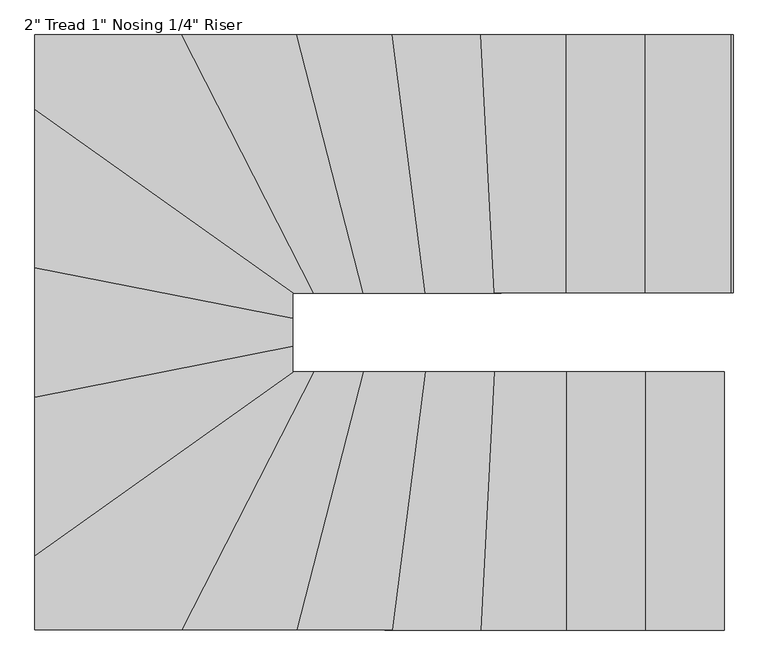
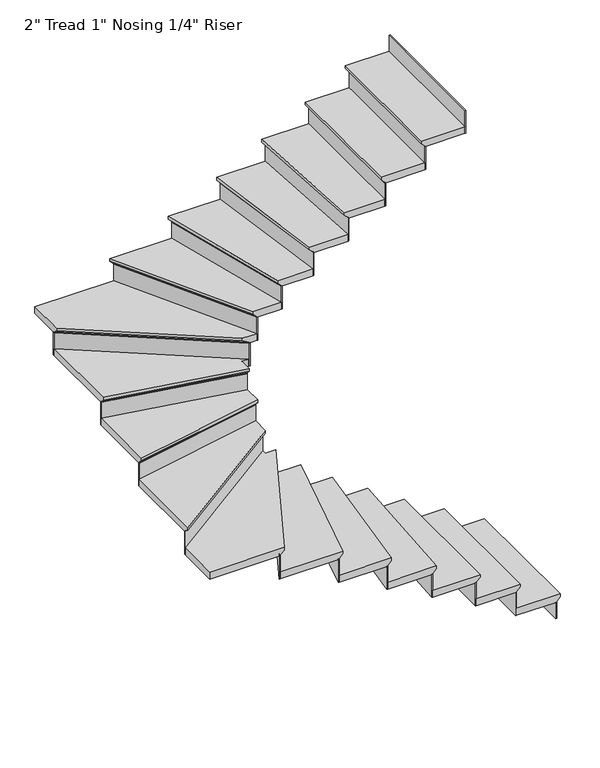
"""IFC4 building model written with IfcOpenShell, lengths in millimetres: stair flight geometry."""

from ifc_helpers import new_model, si_unit, origin, place, context, project, spatial, faceted_brep, source, transform, mapped, element, save


def stair_flight_c61886c8(model_context):
    return source(origin(), model_context, "Body", "Brep", [
        faceted_brep([(-1783.4132248, -345.7070853, 6551.0833333), (-1783.4132248, -345.7070853, 6570.1333333), (-1783.4132248, -1260.1070853, 6570.1333333), (-1783.4132248, -1260.1070853, 6551.0833333), (-1808.8132248, -345.7070853, 6525.6833333), (-1808.8132248, -1260.1070853, 6525.6833333), (-2088.2132248, -345.7070853, 6570.1333333), (-2088.2132248, -1260.1070853, 6570.1333333), (-1808.8132248, -1260.1070853, 6519.3333333), (-2088.2132248, -1260.1070853, 6519.3333333), (-2088.2132248, -345.7070853, 6519.3333333), (-1808.8132248, -345.7070853, 6519.3333333)], [[[0, 1, 2, 3]], [[4, 0, 3, 5]], [[2, 1, 6, 7]], [[8, 9, 10, 11]], [[2, 7, 9, 8, 5, 3]], [[8, 11, 4, 5]], [[6, 1, 0, 4, 11, 10]], [[7, 6, 10, 9]]]),
        faceted_brep([(-1808.8132248, -345.7070853, 6519.3333333), (-1808.8132248, -345.7070853, 6400.8), (-1815.1632248, -345.7070853, 6400.8), (-1815.1632248, -345.7070853, 6519.3333333), (-1808.8132248, -1260.1070853, 6519.3333333), (-1815.1632248, -1260.1070853, 6519.3333333), (-1815.1632248, -1260.1070853, 6400.8), (-1808.8132248, -1260.1070853, 6400.8)], [[[0, 1, 2, 3]], [[4, 5, 6, 7]], [[1, 0, 4, 7]], [[2, 1, 7, 6]], [[3, 2, 6, 5]], [[0, 3, 5, 4]]]),
        faceted_brep([(-2088.2132248, -345.7070853, 6688.6666667), (-2088.2132248, -345.7070853, 6519.3333333), (-2094.5632248, -345.7070853, 6519.3333333), (-2094.5632248, -345.7070853, 6688.6666667), (-2088.2132248, -1260.1070853, 6688.6666667), (-2094.5632248, -1260.1070853, 6688.6666667), (-2094.5632248, -1260.1070853, 6519.3333333), (-2088.2132248, -1260.1070853, 6519.3333333)], [[[0, 1, 2, 3]], [[4, 5, 6, 7]], [[1, 0, 4, 7]], [[2, 1, 7, 6]], [[3, 2, 6, 5]], [[0, 3, 5, 4]]]),
        faceted_brep([(-2062.8132248, -1260.1070853, 6739.4666667), (-2062.8132248, -345.7070853, 6739.4666667), (-2367.6132248, -345.7070853, 6739.4666667), (-2367.6132248, -1260.1070853, 6739.4666667), (-2088.2132248, -1260.1070853, 6688.6666667), (-2367.6132248, -1260.1070853, 6688.6666667), (-2367.6132248, -345.7070853, 6688.6666667), (-2088.2132248, -345.7070853, 6688.6666667), (-2088.2132248, -1260.1070853, 6695.0166667), (-2062.8132248, -1260.1070853, 6720.4166667), (-2088.2132248, -345.7070853, 6695.0166667), (-2062.8132248, -345.7070853, 6720.4166667)], [[[0, 1, 2, 3]], [[4, 5, 6, 7]], [[0, 3, 5, 4, 8, 9]], [[4, 7, 10, 8]], [[2, 1, 11, 10, 7, 6]], [[3, 2, 6, 5]], [[11, 1, 0, 9]], [[10, 11, 9, 8]]]),
        faceted_brep([(-2367.6132248, -345.7070853, 6858.0), (-2367.6132248, -345.7070853, 6688.6666667), (-2373.9632248, -345.7070853, 6688.6666667), (-2373.9632248, -345.7070853, 6858.0), (-2367.6132248, -1260.1070853, 6858.0), (-2373.9632248, -1260.1070853, 6858.0), (-2373.9632248, -1260.1070853, 6688.6666667), (-2367.6132248, -1260.1070853, 6688.6666667)], [[[0, 1, 2, 3]], [[4, 5, 6, 7]], [[1, 0, 4, 7]], [[2, 1, 7, 6]], [[3, 2, 6, 5]], [[0, 3, 5, 4]]]),
        faceted_brep([(-2342.2132248, -1260.1070853, 6908.8), (-2342.2132248, -345.7070853, 6908.8), (-2623.2803863, -345.7070853, 6908.8), (-2670.8146567, -1260.1070853, 6908.8), (-2367.6132248, -1260.1070853, 6858.0), (-2670.8146567, -1260.1070853, 6858.0), (-2623.2803863, -345.7070853, 6858.0), (-2367.6132248, -345.7070853, 6858.0), (-2367.6132248, -1260.1070853, 6864.35), (-2342.2132248, -1260.1070853, 6889.75), (-2367.6132248, -345.7070853, 6864.35), (-2342.2132248, -345.7070853, 6889.75)], [[[0, 1, 2, 3]], [[4, 5, 6, 7]], [[0, 3, 5, 4, 8, 9]], [[4, 7, 10, 8]], [[2, 1, 11, 10, 7, 6]], [[3, 2, 6, 5]], [[11, 1, 0, 9]], [[10, 11, 9, 8]]]),
        faceted_brep([(-2623.2803863, -345.7070853, 7027.3333333), (-2623.2803863, -345.7070853, 6858.0), (-2629.6389604, -345.7070853, 6858.0), (-2629.6389604, -345.7070853, 7027.3333333), (-2670.8146567, -1260.1070853, 7027.3333333), (-2677.1732308, -1260.1070853, 7027.3333333), (-2677.1732308, -1260.1070853, 6858.0), (-2670.8146567, -1260.1070853, 6858.0)], [[[0, 1, 2, 3]], [[4, 5, 6, 7]], [[1, 0, 4, 7]], [[2, 1, 7, 6]], [[3, 2, 6, 5]], [[0, 3, 5, 4]]]),
        faceted_brep([(-2645.38036, -1260.1070853, 7078.1333333), (-2597.8460896, -345.7070853, 7078.1333333), (-2867.4470861, -345.7070853, 7078.1333333), (-2985.8031378, -1260.1070853, 7078.1333333), (-2670.8146567, -1260.1070853, 7027.3333333), (-2985.8031378, -1260.1070853, 7027.3333333), (-2867.4470861, -345.7070853, 7027.3333333), (-2623.2803863, -345.7070853, 7027.3333333), (-2670.8146567, -1260.1070853, 7033.6833333), (-2645.38036, -1260.1070853, 7059.0833333), (-2623.2803863, -345.7070853, 7033.6833333), (-2597.8460896, -345.7070853, 7059.0833333)], [[[0, 1, 2, 3]], [[4, 5, 6, 7]], [[0, 3, 5, 4, 8, 9]], [[4, 7, 10, 8]], [[2, 1, 11, 10, 7, 6]], [[3, 2, 6, 5]], [[11, 1, 0, 9]], [[10, 11, 9, 8]]]),
        faceted_brep([(-2867.4470861, -345.7070853, 7196.6666667), (-2867.4470861, -345.7070853, 7027.3333333), (-2873.8500579, -345.7070853, 7027.3333333), (-2873.8500579, -345.7070853, 7196.6666667), (-2985.8031378, -1260.1070853, 7196.6666667), (-2992.2061095, -1260.1070853, 7196.6666667), (-2992.2061095, -1260.1070853, 7027.3333333), (-2985.8031378, -1260.1070853, 7027.3333333)], [[[0, 1, 2, 3]], [[4, 5, 6, 7]], [[1, 0, 4, 7]], [[2, 1, 7, 6]], [[3, 2, 6, 5]], [[0, 3, 5, 4]]]),
        faceted_brep([(-2960.1912506, -1260.1070853, 7247.4666667), (-2841.835199, -345.7070853, 7247.4666667), (-3089.0743086, -345.7070853, 7247.4666667), (-3324.204756, -1260.1070853, 7247.4666667), (-2985.8031378, -1260.1070853, 7196.6666667), (-3324.204756, -1260.1070853, 7196.6666667), (-3089.0743086, -345.7070853, 7196.6666667), (-2867.4470861, -345.7070853, 7196.6666667), (-2985.8031378, -1260.1070853, 7203.0166667), (-2960.1912506, -1260.1070853, 7228.4166667), (-2867.4470861, -345.7070853, 7203.0166667), (-2841.835199, -345.7070853, 7228.4166667)], [[[0, 1, 2, 3]], [[4, 5, 6, 7]], [[0, 3, 5, 4, 8, 9]], [[4, 7, 10, 8]], [[2, 1, 11, 10, 7, 6]], [[3, 2, 6, 5]], [[11, 1, 0, 9]], [[10, 11, 9, 8]]]),
        faceted_brep([(-3089.0743086, -345.7070853, 7366.0), (-3089.0743086, -345.7070853, 7196.6666667), (-3095.6308854, -345.7070853, 7196.6666667), (-3095.6308854, -345.7070853, 7366.0), (-3324.204756, -1260.1070853, 7366.0), (-3330.7613329, -1260.1070853, 7366.0), (-3330.7613329, -1260.1070853, 7196.6666667), (-3324.204756, -1260.1070853, 7196.6666667)], [[[0, 1, 2, 3]], [[4, 5, 6, 7]], [[1, 0, 4, 7]], [[2, 1, 7, 6]], [[3, 2, 6, 5]], [[0, 3, 5, 4]]]),
        faceted_brep([(-3297.9784485, -1260.1070853, 7416.8), (-3062.8480011, -345.7070853, 7416.8), (-3265.4209447, -345.7070853, 7416.8), (-3734.245566, -1260.1070853, 7416.8), (-3324.204756, -1260.1070853, 7366.0), (-3734.245566, -1260.1070853, 7366.0), (-3265.4209447, -345.7070853, 7366.0), (-3089.0743086, -345.7070853, 7366.0), (-3324.204756, -1260.1070853, 7372.35), (-3297.9784485, -1260.1070853, 7397.75), (-3089.0743086, -345.7070853, 7372.35), (-3062.8480011, -345.7070853, 7397.75)], [[[0, 1, 2, 3]], [[4, 5, 6, 7]], [[0, 3, 5, 4, 8, 9]], [[4, 7, 10, 8]], [[2, 1, 11, 10, 7, 6]], [[3, 2, 6, 5]], [[11, 1, 0, 9]], [[10, 11, 9, 8]]]),
        faceted_brep([(-3265.4209447, -345.7070853, 7535.3333333), (-3265.4209447, -345.7070853, 7366.0), (-3272.5569278, -345.7070853, 7366.0), (-3272.5569278, -345.7070853, 7535.3333333), (-3734.245566, -1260.1070853, 7535.3333333), (-3741.3815491, -1260.1070853, 7535.3333333), (-3741.3815491, -1260.1070853, 7366.0), (-3734.245566, -1260.1070853, 7366.0)], [[[0, 1, 2, 3]], [[4, 5, 6, 7]], [[1, 0, 4, 7]], [[2, 1, 7, 6]], [[3, 2, 6, 5]], [[0, 3, 5, 4]]]),
        faceted_brep([(-4225.5449167, -966.4259516, 7586.1333333), (-4225.5449167, -1260.1070853, 7586.1333333), (-3705.7016335, -1260.1070853, 7586.1333333), (-3236.8770121, -345.7070853, 7586.1333333), (-3311.1449167, -345.7070853, 7586.1333333), (-3311.1449167, -316.1520025, 7586.1333333), (-4225.5449167, -1260.1070853, 7535.3333333), (-4225.5449167, -966.4259516, 7535.3333333), (-3311.1449167, -316.1520025, 7535.3333333), (-3311.1449167, -345.7070853, 7535.3333333), (-3265.4209447, -345.7070853, 7535.3333333), (-3734.245566, -1260.1070853, 7535.3333333), (-3734.245566, -1260.1070853, 7541.6833333), (-3705.7016335, -1260.1070853, 7567.0833333), (-3265.4209447, -345.7070853, 7541.6833333), (-3236.8770121, -345.7070853, 7567.0833333)], [[[0, 1, 2, 3, 4, 5]], [[6, 7, 8, 9, 10, 11]], [[1, 0, 7, 6]], [[2, 1, 6, 11, 12, 13]], [[11, 10, 14, 12]], [[4, 3, 15, 14, 10, 9]], [[5, 4, 9, 8]], [[0, 5, 8, 7]], [[15, 3, 2, 13]], [[14, 15, 13, 12]]]),
        faceted_brep([(-3311.1449167, -316.1520025, 7704.6666667), (-3311.1449167, -316.1520025, 7535.3333333), (-3311.1449167, -308.3600277, 7535.3333333), (-3311.1449167, -308.3600277, 7704.6666667), (-4225.5449167, -966.4259516, 7704.6666667), (-4225.5449167, -958.6339768, 7704.6666667), (-4225.5449167, -958.6339768, 7535.3333333), (-4225.5449167, -966.4259516, 7535.3333333)], [[[0, 1, 2, 3]], [[4, 5, 6, 7]], [[1, 0, 4, 7]], [[2, 1, 7, 6]], [[3, 2, 6, 5]], [[0, 3, 5, 4]]]),
        faceted_brep([(-4225.5449167, -997.5938508, 7755.4666667), (-3311.1449167, -347.3199017, 7755.4666667), (-3311.1449167, -229.6979154, 7755.4666667), (-4225.5449167, -409.9387717, 7755.4666667), (-4225.5449167, -966.4259516, 7704.6666667), (-4225.5449167, -409.9387717, 7704.6666667), (-3311.1449167, -229.6979154, 7704.6666667), (-3311.1449167, -316.1520025, 7704.6666667), (-4225.5449167, -966.4259516, 7711.0166667), (-4225.5449167, -997.5938508, 7736.4166667), (-3311.1449167, -316.1520025, 7711.0166667), (-3311.1449167, -347.3199017, 7736.4166667)], [[[0, 1, 2, 3]], [[4, 5, 6, 7]], [[0, 3, 5, 4, 8, 9]], [[4, 7, 10, 8]], [[2, 1, 11, 10, 7, 6]], [[3, 2, 6, 5]], [[11, 1, 0, 9]], [[10, 11, 9, 8]]]),
        faceted_brep([(-3311.1449167, -229.6979154, 7874.0), (-3311.1449167, -229.6979154, 7704.6666667), (-3311.1449167, -223.22573, 7704.6666667), (-3311.1449167, -223.22573, 7874.0), (-4225.5449167, -409.9387717, 7874.0), (-4225.5449167, -403.4665863, 7874.0), (-4225.5449167, -403.4665863, 7704.6666667), (-4225.5449167, -409.9387717, 7704.6666667)], [[[0, 1, 2, 3]], [[4, 5, 6, 7]], [[1, 0, 4, 7]], [[2, 1, 7, 6]], [[3, 2, 6, 5]], [[0, 3, 5, 4]]]),
        faceted_brep([(-4225.5449167, -435.8275135, 7924.8), (-3311.1449167, -255.5866572, 7924.8), (-3311.1449167, -130.5387717, 7924.8), (-4225.5449167, 49.7020846, 7924.8), (-4225.5449167, -409.9387717, 7874.0), (-4225.5449167, 49.7020846, 7874.0), (-3311.1449167, -130.5387717, 7874.0), (-3311.1449167, -229.6979154, 7874.0), (-4225.5449167, -409.9387717, 7880.35), (-4225.5449167, -435.8275135, 7905.75), (-3311.1449167, -229.6979154, 7880.35), (-3311.1449167, -255.5866572, 7905.75)], [[[0, 1, 2, 3]], [[4, 5, 6, 7]], [[0, 3, 5, 4, 8, 9]], [[4, 7, 10, 8]], [[2, 1, 11, 10, 7, 6]], [[3, 2, 6, 5]], [[11, 1, 0, 9]], [[10, 11, 9, 8]]]),
        faceted_brep([(-3311.1449167, -130.5387717, 8043.3333333), (-3311.1449167, -130.5387717, 7874.0), (-3311.1449167, -124.0665863, 7874.0), (-3311.1449167, -124.0665863, 8043.3333333), (-4225.5449167, 49.7020846, 8043.3333333), (-4225.5449167, 56.17427, 8043.3333333), (-4225.5449167, 56.17427, 7874.0), (-4225.5449167, 49.7020846, 7874.0)], [[[0, 1, 2, 3]], [[4, 5, 6, 7]], [[1, 0, 4, 7]], [[2, 1, 7, 6]], [[3, 2, 6, 5]], [[0, 3, 5, 4]]]),
        faceted_brep([(-4225.5449167, 23.8133428, 8094.1333333), (-3311.1449167, -156.4275135, 8094.1333333), (-3311.1449167, -66.3070853, 8094.1333333), (-3265.0494422, -66.3070853, 8094.1333333), (-4225.5449167, 616.7475793, 8094.1333333), (-4225.5449167, 49.7020846, 8043.3333333), (-4225.5449167, 616.7475793, 8043.3333333), (-3265.0494422, -66.3070853, 8043.3333333), (-3311.1449167, -66.3070853, 8043.3333333), (-3311.1449167, -130.5387717, 8043.3333333), (-4225.5449167, 49.7020846, 8049.6833333), (-4225.5449167, 23.8133428, 8075.0833333), (-3311.1449167, -130.5387717, 8049.6833333), (-3311.1449167, -156.4275135, 8075.0833333)], [[[0, 1, 2, 3, 4]], [[5, 6, 7, 8, 9]], [[0, 4, 6, 5, 10, 11]], [[5, 9, 12, 10]], [[2, 1, 13, 12, 9, 8]], [[3, 2, 8, 7]], [[4, 3, 7, 6]], [[13, 1, 0, 11]], [[12, 13, 11, 10]]]),
        faceted_brep([(-3265.0494422, -66.3070853, 8212.6666667), (-3265.0494422, -66.3070853, 8043.3333333), (-3254.0925497, -66.3070853, 8043.3333333), (-3254.0925497, -66.3070853, 8212.6666667), (-4225.5449167, 616.7475793, 8212.6666667), (-4225.5449167, 624.5395541, 8212.6666667), (-4225.5449167, 624.5395541, 8043.3333333), (-4225.5449167, 616.7475793, 8043.3333333)], [[[0, 1, 2, 3]], [[4, 5, 6, 7]], [[1, 0, 4, 7]], [[2, 1, 7, 6]], [[3, 2, 6, 5]], [[0, 3, 5, 4]]]),
        faceted_brep([(-3677.1577009, 848.0929147, 8263.4666667), (-4225.5449167, 848.0929147, 8263.4666667), (-4225.5449167, 585.5796802, 8263.4666667), (-3308.8770121, -66.3070853, 8263.4666667), (-3208.3330796, -66.3070853, 8263.4666667), (-4225.5449167, 848.0929147, 8212.6666667), (-3677.1577009, 848.0929147, 8212.6666667), (-3208.3330796, -66.3070853, 8212.6666667), (-3265.0494422, -66.3070853, 8212.6666667), (-4225.5449167, 616.7475793, 8212.6666667), (-4225.5449167, 616.7475793, 8219.0166667), (-4225.5449167, 585.5796802, 8244.4166667), (-3265.0494422, -66.3070853, 8219.0166667), (-3308.8770121, -66.3070853, 8244.4166667)], [[[0, 1, 2, 3, 4]], [[5, 6, 7, 8, 9]], [[1, 0, 6, 5]], [[2, 1, 5, 9, 10, 11]], [[9, 8, 12, 10]], [[4, 3, 13, 12, 8, 7]], [[0, 4, 7, 6]], [[13, 3, 2, 11]], [[12, 13, 11, 10]]]),
        faceted_brep([(-3208.3330796, -66.3070853, 8382.0), (-3208.3330796, -66.3070853, 8212.6666667), (-3201.1970965, -66.3070853, 8212.6666667), (-3201.1970965, -66.3070853, 8382.0), (-3677.1577009, 848.0929147, 8382.0), (-3670.0217178, 848.0929147, 8382.0), (-3670.0217178, 848.0929147, 8212.6666667), (-3677.1577009, 848.0929147, 8212.6666667)], [[[0, 1, 2, 3]], [[4, 5, 6, 7]], [[1, 0, 4, 7]], [[2, 1, 7, 6]], [[3, 2, 6, 5]], [[0, 3, 5, 4]]]),
        faceted_brep([(-3705.7016335, 848.0929147, 8432.8), (-3236.8770121, -66.3070853, 8432.8), (-3036.6216937, -66.3070853, 8432.8), (-3271.7521411, 848.0929147, 8432.8), (-3677.1577009, 848.0929147, 8382.0), (-3271.7521411, 848.0929147, 8382.0), (-3036.6216937, -66.3070853, 8382.0), (-3208.3330796, -66.3070853, 8382.0), (-3677.1577009, 848.0929147, 8388.35), (-3705.7016335, 848.0929147, 8413.75), (-3208.3330796, -66.3070853, 8388.35), (-3236.8770121, -66.3070853, 8413.75)], [[[0, 1, 2, 3]], [[4, 5, 6, 7]], [[0, 3, 5, 4, 8, 9]], [[4, 7, 10, 8]], [[2, 1, 11, 10, 7, 6]], [[3, 2, 6, 5]], [[11, 1, 0, 9]], [[10, 11, 9, 8]]]),
        faceted_brep([(-3036.6216937, -66.3070853, 8551.3333333), (-3036.6216937, -66.3070853, 8382.0), (-3030.0651168, -66.3070853, 8382.0), (-3030.0651168, -66.3070853, 8551.3333333), (-3271.7521411, 848.0929147, 8551.3333333), (-3265.1955642, 848.0929147, 8551.3333333), (-3265.1955642, 848.0929147, 8382.0), (-3271.7521411, 848.0929147, 8382.0)], [[[0, 1, 2, 3]], [[4, 5, 6, 7]], [[1, 0, 4, 7]], [[2, 1, 7, 6]], [[3, 2, 6, 5]], [[0, 3, 5, 4]]]),
        faceted_brep([(-3297.9784485, 848.0929147, 8602.1333333), (-3062.8480011, -66.3070853, 8602.1333333), (-2816.2233119, -66.3070853, 8602.1333333), (-2934.5793635, 848.0929147, 8602.1333333), (-3271.7521411, 848.0929147, 8551.3333333), (-2934.5793635, 848.0929147, 8551.3333333), (-2816.2233119, -66.3070853, 8551.3333333), (-3036.6216937, -66.3070853, 8551.3333333), (-3271.7521411, 848.0929147, 8557.6833333), (-3297.9784485, 848.0929147, 8583.0833333), (-3036.6216937, -66.3070853, 8557.6833333), (-3062.8480011, -66.3070853, 8583.0833333)], [[[0, 1, 2, 3]], [[4, 5, 6, 7]], [[0, 3, 5, 4, 8, 9]], [[4, 7, 10, 8]], [[2, 1, 11, 10, 7, 6]], [[3, 2, 6, 5]], [[11, 1, 0, 9]], [[10, 11, 9, 8]]]),
        faceted_brep([(-2816.2233119, -66.3070853, 8720.6666667), (-2816.2233119, -66.3070853, 8551.3333333), (-2809.8203401, -66.3070853, 8551.3333333), (-2809.8203401, -66.3070853, 8720.6666667), (-2934.5793635, 848.0929147, 8720.6666667), (-2928.1763918, 848.0929147, 8720.6666667), (-2928.1763918, 848.0929147, 8551.3333333), (-2934.5793635, 848.0929147, 8551.3333333)], [[[0, 1, 2, 3]], [[4, 5, 6, 7]], [[1, 0, 4, 7]], [[2, 1, 7, 6]], [[3, 2, 6, 5]], [[0, 3, 5, 4]]]),
        faceted_brep([(-2960.1912506, 848.0929147, 8771.4666667), (-2841.835199, -66.3070853, 8771.4666667), (-2572.411793, -66.3070853, 8771.4666667), (-2619.9460634, 848.0929147, 8771.4666667), (-2934.5793635, 848.0929147, 8720.6666667), (-2619.9460634, 848.0929147, 8720.6666667), (-2572.411793, -66.3070853, 8720.6666667), (-2816.2233119, -66.3070853, 8720.6666667), (-2934.5793635, 848.0929147, 8727.0166667), (-2960.1912506, 848.0929147, 8752.4166667), (-2816.2233119, -66.3070853, 8727.0166667), (-2841.835199, -66.3070853, 8752.4166667)], [[[0, 1, 2, 3]], [[4, 5, 6, 7]], [[0, 3, 5, 4, 8, 9]], [[4, 7, 10, 8]], [[2, 1, 11, 10, 7, 6]], [[3, 2, 6, 5]], [[11, 1, 0, 9]], [[10, 11, 9, 8]]]),
        faceted_brep([(-2572.411793, -66.3070853, 8890.0), (-2572.411793, -66.3070853, 8720.6666667), (-2566.0532188, -66.3070853, 8720.6666667), (-2566.0532188, -66.3070853, 8890.0), (-2619.9460634, 848.0929147, 8890.0), (-2613.5874892, 848.0929147, 8890.0), (-2613.5874892, 848.0929147, 8720.6666667), (-2619.9460634, 848.0929147, 8720.6666667)], [[[0, 1, 2, 3]], [[4, 5, 6, 7]], [[1, 0, 4, 7]], [[2, 1, 7, 6]], [[3, 2, 6, 5]], [[0, 3, 5, 4]]]),
        faceted_brep([(-2645.38036, 848.0929147, 8940.8), (-2597.8460896, -66.3070853, 8940.8), (-2316.8132248, -66.3070853, 8940.8), (-2316.8132248, 848.0929147, 8940.8), (-2619.9460634, 848.0929147, 8890.0), (-2316.8132248, 848.0929147, 8890.0), (-2316.8132248, -66.3070853, 8890.0), (-2572.411793, -66.3070853, 8890.0), (-2619.9460634, 848.0929147, 8896.35), (-2645.38036, 848.0929147, 8921.75), (-2572.411793, -66.3070853, 8896.35), (-2597.8460896, -66.3070853, 8921.75)], [[[0, 1, 2, 3]], [[4, 5, 6, 7]], [[0, 3, 5, 4, 8, 9]], [[4, 7, 10, 8]], [[2, 1, 11, 10, 7, 6]], [[3, 2, 6, 5]], [[11, 1, 0, 9]], [[10, 11, 9, 8]]]),
        faceted_brep([(-2316.8132248, -66.3070853, 9059.3333333), (-2316.8132248, -66.3070853, 8890.0), (-2310.4632248, -66.3070853, 8890.0), (-2310.4632248, -66.3070853, 9059.3333333), (-2316.8132248, 848.0929147, 9059.3333333), (-2310.4632248, 848.0929147, 9059.3333333), (-2310.4632248, 848.0929147, 8890.0), (-2316.8132248, 848.0929147, 8890.0)], [[[0, 1, 2, 3]], [[4, 5, 6, 7]], [[1, 0, 4, 7]], [[2, 1, 7, 6]], [[3, 2, 6, 5]], [[0, 3, 5, 4]]]),
        faceted_brep([(-2342.2132248, 848.0929147, 9110.1333333), (-2342.2132248, -66.3070853, 9110.1333333), (-2037.4132248, -66.3070853, 9110.1333333), (-2037.4132248, 848.0929147, 9110.1333333), (-2316.8132248, 848.0929147, 9059.3333333), (-2037.4132248, 848.0929147, 9059.3333333), (-2037.4132248, -66.3070853, 9059.3333333), (-2316.8132248, -66.3070853, 9059.3333333), (-2316.8132248, 848.0929147, 9065.6833333), (-2342.2132248, 848.0929147, 9091.0833333), (-2316.8132248, -66.3070853, 9065.6833333), (-2342.2132248, -66.3070853, 9091.0833333)], [[[0, 1, 2, 3]], [[4, 5, 6, 7]], [[0, 3, 5, 4, 8, 9]], [[4, 7, 10, 8]], [[2, 1, 11, 10, 7, 6]], [[3, 2, 6, 5]], [[11, 1, 0, 9]], [[10, 11, 9, 8]]]),
        faceted_brep([(-2037.4132248, -66.3070853, 9228.6666667), (-2037.4132248, -66.3070853, 9059.3333333), (-2031.0632248, -66.3070853, 9059.3333333), (-2031.0632248, -66.3070853, 9228.6666667), (-2037.4132248, 848.0929147, 9228.6666667), (-2031.0632248, 848.0929147, 9228.6666667), (-2031.0632248, 848.0929147, 9059.3333333), (-2037.4132248, 848.0929147, 9059.3333333)], [[[0, 1, 2, 3]], [[4, 5, 6, 7]], [[1, 0, 4, 7]], [[2, 1, 7, 6]], [[3, 2, 6, 5]], [[0, 3, 5, 4]]]),
        faceted_brep([(-1758.0132248, -66.3070853, 9398.0), (-1758.0132248, -66.3070853, 9228.6666667), (-1751.6632248, -66.3070853, 9228.6666667), (-1751.6632248, -66.3070853, 9398.0), (-1758.0132248, 848.0929147, 9398.0), (-1751.6632248, 848.0929147, 9398.0), (-1751.6632248, 848.0929147, 9228.6666667), (-1758.0132248, 848.0929147, 9228.6666667)], [[[0, 1, 2, 3]], [[4, 5, 6, 7]], [[1, 0, 4, 7]], [[2, 1, 7, 6]], [[3, 2, 6, 5]], [[0, 3, 5, 4]]]),
        faceted_brep([(-2062.8132248, 848.0929147, 9279.4666667), (-2062.8132248, -66.3070853, 9279.4666667), (-1758.0132248, -66.3070853, 9279.4666667), (-1758.0132248, 848.0929147, 9279.4666667), (-2037.4132248, 848.0929147, 9228.6666667), (-1758.0132248, 848.0929147, 9228.6666667), (-1758.0132248, -66.3070853, 9228.6666667), (-2037.4132248, -66.3070853, 9228.6666667), (-2037.4132248, 848.0929147, 9235.0166667), (-2062.8132248, 848.0929147, 9260.4166667), (-2037.4132248, -66.3070853, 9235.0166667), (-2062.8132248, -66.3070853, 9260.4166667)], [[[0, 1, 2, 3]], [[4, 5, 6, 7]], [[0, 3, 5, 4, 8, 9]], [[4, 7, 10, 8]], [[2, 1, 11, 10, 7, 6]], [[3, 2, 6, 5]], [[11, 1, 0, 9]], [[10, 11, 9, 8]]]),
    ])


if __name__ == "__main__":
    model = new_model("IFC4")
    model_context = context("Model", 3, world=origin())
    ifc_project = project(units=[si_unit("LENGTHUNIT", "METRE", prefix="MILLI")], contexts=[model_context])
    site = spatial("IfcSite", under=ifc_project)
    building = spatial("IfcBuilding", under=site)
    placement = place(None, origin())
    stair_flight_shape = stair_flight_c61886c8(model_context)
    element("IfcStairFlight", 1, ObjectType="2\" Tread 1\" Nosing 1/4\" Riser", at=placement, inside=building, context=model_context, shape_type="MappedRepresentation", body=[
        mapped(stair_flight_shape, transform((0.0, 0.0, 0.0), x_axis=(1.0, 0.0, 0.0), y_axis=(0.0, 1.0, 0.0), z_axis=(0.0, 0.0, 1.0))),
    ])
    save(model, "model.ifc")
